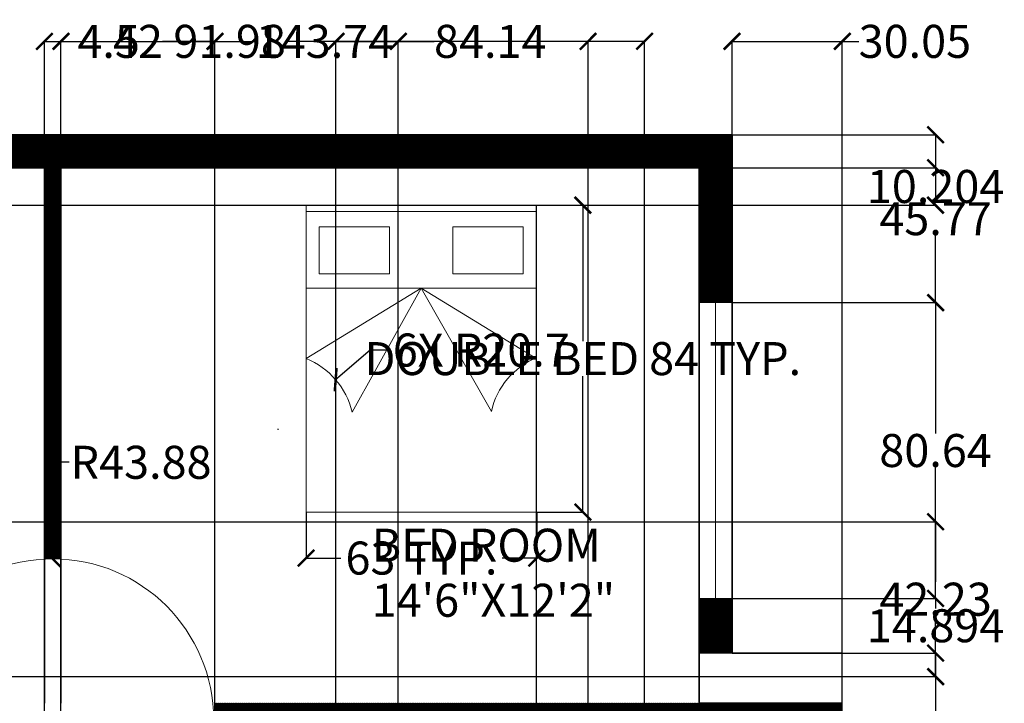
# Model space of a CAD drawing. Units: inches. Extents: x -43 to 552, y 22 to 537.
# Tile 4 of 4: x 283 to 552, y 351 to 537. Entities that reach past the tile are written whole.
import ezdxf

# ---------------------------------------------------------------- set-up
doc = ezdxf.new("R2010")
doc.units = ezdxf.units.IN
doc.header["$MEASUREMENT"] = 0
for name, color, linetype, lineweight in [('A-ANNO-DIMS', 2, 'Continuous', 18), ('A-AREA-IDEN', 7, 'Continuous', 18), ('A-DOOR', 4, 'Continuous', 18), ('A-FLOR', 7, 'Continuous', 25), ('A-FURN', 8, 'Continuous', 18), ('A-GLAZ', 4, 'Continuous', 18), ('A-WALL', 7, 'Continuous', 35), ('A-WALL-PATT', 252, 'Continuous', 13)]:
    doc.layers.add(name, color=color, linetype=linetype, lineweight=lineweight)
doc.styles.get("Standard").update_dxf_attribs({"font": 'arial.ttf'})
doc.dimstyles.get("Standard").update_dxf_attribs({"dimtxt": 9, "dimasz": 4.5, "dimexe": 0.18, "dimexo": 0.0625, "dimgap": 0.09, "dimtad": 0, "dimtih": 1, "dimtoh": 1, "dimdec": 1, "dimzin": 0, "dimdsep": 46, "dimlunit": 4, "dimtxsty": 'Standard', "dimblk": 'ARCHTICK', "dimcen": 0.09, "dimadec": 0, "dimazin": 0, "dimtfac": 1, "dimtdec": 1, "dimtofl": 0, "dimtmove": 0, "dimatfit": 3, "dimfxl": 1, "dimtolj": 1, "dimtzin": 0, "dimarcsym": 0})
pattern_1 = [(45, (-523.11303, 0), (-0.088388348, 0.088388348), [])]

# ---------------------------------------------------------------- blocks, each defined once
blk = doc.blocks.new('BED-DOUBLE')
for p, q in [((0, 83.65), (62.74, 83.65)), ((0, 0), (0, 83.65)), ((62.74, 83.65), (62.74, 0)), ((0, 81.91), (62.74, 81.91)), ((0, 61), (62.74, 61)), ((31.37, 61), (0, 41.83)), ((12.53, 27.23), (31.37, 61)), ((62.74, 41.83), (31.37, 61)), ((31.37, 61), (50.51, 27.4)), ((62.74, 0), (0, 0))]:
    blk.add_line(p, q)
for points in [[(3.55, 77.79), (22.76, 77.79), (22.76, 64.95), (3.55, 64.95)], [(59.19, 77.79), (39.98, 77.79), (39.98, 64.95), (59.19, 64.95)]]:
    blk.add_lwpolyline(points, close=True)
for centre, start, end in [((-7.65, 22.59), 12.9482, 68.3142), ((70.73, 22.94), 112.1918, 167.5578)]:
    blk.add_arc(centre, 20.7, start, end)
blk = doc.blocks.new('_ArchTick')
at = {"color": 0, "linetype": 'ByBlock', "const_width": 0.15}
blk.add_lwpolyline([(-0.5, -0.5), (0.5, 0.5)], dxfattribs=at)
blk = doc.blocks.new('*D4')
at = {"layer": 'A-ANNO-DIMS', "color": 0, "lineweight": -2, "transparency": 16777216}
for p, q in [((424.33, 486.74), (437, 486.74)), ((436.82, 486.74), (436.82, 449.66)), ((436.82, 403.09), (436.82, 440.17)), ((424.33, 403.09), (437, 403.09))]:
    blk.add_line(p, q, dxfattribs=at)
at = {"layer": 'Defpoints', "color": 0, "transparency": 16777216}
for p in [(424.27, 486.74), (436.82, 486.74), (424.27, 403.09)]:
    blk.add_point(p, dxfattribs=at)
at = {"layer": 'A-ANNO-DIMS', "color": 0, "lineweight": -2, "transparency": 16777216, "xscale": 4.5, "yscale": 4.5, "zscale": 4.5}
for p, rotation in [((436.82, 486.74), 90), ((436.82, 403.09), 270)]:
    blk.add_blockref('_ArchTick', p, dxfattribs=dict(at, rotation=rotation))
at = {"layer": 'A-ANNO-DIMS', "color": 0, "transparency": 16777216, "insert": (436.82, 444.92), "char_height": 9, "attachment_point": 5}
blk.add_mtext('\\A1;DOUBLE BED 84 TYP.', dxfattribs=at)
blk = doc.blocks.new('*D5')
at = {"layer": 'A-ANNO-DIMS', "color": 0, "lineweight": -2, "transparency": 16777216}
for p, q in [((361.36, 403.03), (361.36, 390.36)), ((424.27, 403.03), (424.27, 390.36)), ((361.36, 390.54), (370.8, 390.54)), ((424.27, 390.54), (414.84, 390.54))]:
    blk.add_line(p, q, dxfattribs=at)
at = {"layer": 'Defpoints', "color": 0, "transparency": 16777216}
for p in [(361.36, 403.09), (424.27, 403.09), (424.27, 390.54)]:
    blk.add_point(p, dxfattribs=at)
at = {"layer": 'A-ANNO-DIMS', "color": 0, "lineweight": -2, "transparency": 16777216, "xscale": 4.5, "yscale": 4.5, "zscale": 4.5, "rotation": 180}
blk.add_blockref('_ArchTick', (361.36, 390.54), dxfattribs=at)
at = {"layer": 'A-ANNO-DIMS', "color": 0, "lineweight": -2, "transparency": 16777216, "xscale": 4.5, "yscale": 4.5, "zscale": 4.5}
blk.add_blockref('_ArchTick', (424.27, 390.54), dxfattribs=at)
at = {"layer": 'A-ANNO-DIMS', "color": 0, "transparency": 16777216, "insert": (392.82, 390.54), "char_height": 9, "attachment_point": 5}
blk.add_mtext('\\A1;63 TYP.', dxfattribs=at)
blk = doc.blocks.new('*D9')
at = {"layer": 'A-ANNO-DIMS', "color": 0, "lineweight": -2, "transparency": 16777216}
for p, q in [((82.45, 505.95), (-24.17, 505.95)), ((-23.99, 505.95), (-23.99, 287.55)), ((-23.99, 59.77), (-23.99, 278.18)), ((289.95, 59.77), (-24.17, 59.77))]:
    blk.add_line(p, q, dxfattribs=at)
at = {"layer": 'Defpoints', "color": 0, "transparency": 16777216}
for p in [(-23.99, 505.95), (82.51, 505.95), (290.01, 59.77)]:
    blk.add_point(p, dxfattribs=at)
at = {"layer": 'A-ANNO-DIMS', "color": 0, "lineweight": -2, "transparency": 16777216, "xscale": 4.5, "yscale": 4.5, "zscale": 4.5}
for p, rotation in [((-23.99, 505.95), 90), ((-23.99, 59.77), 270)]:
    blk.add_blockref('_ArchTick', p, dxfattribs=dict(at, rotation=rotation))
at = {"layer": 'A-ANNO-DIMS', "color": 0, "transparency": 16777216, "insert": (-23.99, 282.86), "char_height": 9, "attachment_point": 5}
blk.add_mtext('\\A1;446.2', dxfattribs=at)
blk = doc.blocks.new('*D15')
at = {"layer": 'A-ANNO-DIMS', "color": 0, "lineweight": -2, "transparency": 16777216}
for p, q in [((477.51, 506.01), (477.51, 531.58)), ((477.51, 531.4), (507.56, 531.4)), ((507.56, 364.71), (507.56, 531.58)), ((507.56, 531.4), (512.06, 531.4))]:
    blk.add_line(p, q, dxfattribs=at)
at = {"layer": 'Defpoints', "color": 0, "transparency": 16777216}
for p in [(507.56, 531.4), (477.51, 505.95), (507.56, 364.65)]:
    blk.add_point(p, dxfattribs=at)
at = {"layer": 'A-ANNO-DIMS', "color": 0, "lineweight": -2, "transparency": 16777216, "xscale": 4.5, "yscale": 4.5, "zscale": 4.5, "rotation": 180}
blk.add_blockref('_ArchTick', (477.51, 531.4), dxfattribs=at)
at = {"layer": 'A-ANNO-DIMS', "color": 0, "lineweight": -2, "transparency": 16777216, "xscale": 4.5, "yscale": 4.5, "zscale": 4.5}
blk.add_blockref('_ArchTick', (507.56, 531.4), dxfattribs=at)
at = {"layer": 'A-ANNO-DIMS', "color": 0, "transparency": 16777216, "insert": (527.37, 531.4), "char_height": 9, "attachment_point": 5}
blk.add_mtext('\\A1;30.05', dxfattribs=at)
blk = doc.blocks.new('*D16')
at = {"layer": 'A-ANNO-DIMS', "color": 0, "lineweight": -2, "transparency": 16777216}
for p, q in [((477.57, 460.18), (533.19, 460.18)), ((533.01, 460.18), (533.01, 424.54)), ((533.01, 379.54), (533.01, 415.17)), ((477.57, 379.54), (533.19, 379.54))]:
    blk.add_line(p, q, dxfattribs=at)
at = {"layer": 'Defpoints', "color": 0, "transparency": 16777216}
for p in [(477.51, 460.18), (533.01, 460.18), (477.51, 379.54)]:
    blk.add_point(p, dxfattribs=at)
at = {"layer": 'A-ANNO-DIMS', "color": 0, "lineweight": -2, "transparency": 16777216, "xscale": 4.5, "yscale": 4.5, "zscale": 4.5}
for p, rotation in [((533.01, 460.18), 90), ((533.01, 379.54), 270)]:
    blk.add_blockref('_ArchTick', p, dxfattribs=dict(at, rotation=rotation))
at = {"layer": 'A-ANNO-DIMS', "color": 0, "transparency": 16777216, "insert": (533.01, 419.86), "char_height": 9, "attachment_point": 5}
blk.add_mtext('\\A1;80.64', dxfattribs=at)
blk = doc.blocks.new('*D17')
at = {"layer": 'A-ANNO-DIMS', "color": 0, "lineweight": -2, "transparency": 16777216}
for p, q in [((477.57, 505.95), (533.19, 505.95)), ((533.01, 505.95), (533.01, 487.73)), ((533.01, 460.18), (533.01, 478.39)), ((477.57, 460.18), (533.19, 460.18))]:
    blk.add_line(p, q, dxfattribs=at)
at = {"layer": 'Defpoints', "color": 0, "transparency": 16777216}
for p in [(477.51, 505.95), (533.01, 505.95), (477.51, 460.18)]:
    blk.add_point(p, dxfattribs=at)
at = {"layer": 'A-ANNO-DIMS', "color": 0, "lineweight": -2, "transparency": 16777216, "xscale": 4.5, "yscale": 4.5, "zscale": 4.5}
for p, rotation in [((533.01, 505.95), 90), ((533.01, 460.18), 270)]:
    blk.add_blockref('_ArchTick', p, dxfattribs=dict(at, rotation=rotation))
at = {"layer": 'A-ANNO-DIMS', "color": 0, "transparency": 16777216, "insert": (533.01, 483.06), "char_height": 9, "attachment_point": 5}
blk.add_mtext('\\A1;45.77', dxfattribs=at)
blk = doc.blocks.new('*D18')
at = {"layer": 'A-ANNO-DIMS', "color": 0, "lineweight": -2, "transparency": 16777216}
for p, q in [((477.57, 379.54), (533.19, 379.54)), ((533.01, 379.54), (533.01, 376.78)), ((533.01, 364.65), (533.01, 367.41)), ((477.57, 364.65), (533.19, 364.65))]:
    blk.add_line(p, q, dxfattribs=at)
at = {"layer": 'Defpoints', "color": 0, "transparency": 16777216}
for p in [(477.51, 379.54), (533.01, 379.54), (477.51, 364.65)]:
    blk.add_point(p, dxfattribs=at)
at = {"layer": 'A-ANNO-DIMS', "color": 0, "lineweight": -2, "transparency": 16777216, "xscale": 4.5, "yscale": 4.5, "zscale": 4.5}
for p, rotation in [((533.01, 379.54), 90), ((533.01, 364.65), 270)]:
    blk.add_blockref('_ArchTick', p, dxfattribs=dict(at, rotation=rotation))
at = {"layer": 'A-ANNO-DIMS', "color": 0, "transparency": 16777216, "insert": (533.01, 372.09), "char_height": 9, "attachment_point": 5}
blk.add_mtext('\\A1;14.894', dxfattribs=at)
blk = doc.blocks.new('*D19')
at = {"layer": 'A-ANNO-DIMS', "color": 0, "lineweight": -2, "transparency": 16777216}
for p, q in [((507.62, 364.65), (533.19, 364.65)), ((533.01, 364.65), (533.01, 297.15)), ((533.01, 220.29), (533.01, 287.78)), ((507.62, 220.29), (533.19, 220.29))]:
    blk.add_line(p, q, dxfattribs=at)
at = {"layer": 'Defpoints', "color": 0, "transparency": 16777216}
for p in [(507.56, 364.65), (533.01, 364.65), (507.56, 220.29)]:
    blk.add_point(p, dxfattribs=at)
at = {"layer": 'A-ANNO-DIMS', "color": 0, "lineweight": -2, "transparency": 16777216, "xscale": 4.5, "yscale": 4.5, "zscale": 4.5}
for p, rotation in [((533.01, 364.65), 90), ((533.01, 220.29), 270)]:
    blk.add_blockref('_ArchTick', p, dxfattribs=dict(at, rotation=rotation))
at = {"layer": 'A-ANNO-DIMS', "color": 0, "transparency": 16777216, "insert": (533.01, 292.47), "char_height": 9, "attachment_point": 5}
blk.add_mtext('\\A1;144.36', dxfattribs=at)
blk = doc.blocks.new('*D28')
at = {"layer": 'A-ANNO-DIMS', "color": 0, "lineweight": -2, "transparency": 16777216}
for p, q in [((369.51, 297.17), (369.51, 531.58)), ((369.51, 531.4), (396.32, 531.4)), ((453.65, 531.4), (426.84, 531.4)), ((453.65, 297.17), (453.65, 531.58))]:
    blk.add_line(p, q, dxfattribs=at)
at = {"layer": 'Defpoints', "color": 0, "transparency": 16777216}
for p in [(453.65, 531.4), (369.51, 297.11), (453.65, 297.11)]:
    blk.add_point(p, dxfattribs=at)
at = {"layer": 'A-ANNO-DIMS', "color": 0, "lineweight": -2, "transparency": 16777216, "xscale": 4.5, "yscale": 4.5, "zscale": 4.5, "rotation": 180}
blk.add_blockref('_ArchTick', (369.51, 531.4), dxfattribs=at)
at = {"layer": 'A-ANNO-DIMS', "color": 0, "lineweight": -2, "transparency": 16777216, "xscale": 4.5, "yscale": 4.5, "zscale": 4.5}
blk.add_blockref('_ArchTick', (453.65, 531.4), dxfattribs=at)
at = {"layer": 'A-ANNO-DIMS', "color": 0, "transparency": 16777216, "insert": (411.58, 531.4), "char_height": 9, "attachment_point": 5}
blk.add_mtext('\\A1;84.14', dxfattribs=at)
blk = doc.blocks.new('*D32')
at = {"layer": 'A-ANNO-DIMS', "color": 0, "lineweight": -2, "transparency": 16777216}
for p, q in [((290.01, 255.18), (290.01, 531.58)), ((290.01, 531.4), (294.51, 531.4)), ((294.51, 255.18), (294.51, 531.58)), ((294.51, 531.4), (299.01, 531.4))]:
    blk.add_line(p, q, dxfattribs=at)
at = {"layer": 'Defpoints', "color": 0, "transparency": 16777216}
for p in [(294.51, 531.4), (290.01, 255.12), (294.51, 255.12)]:
    blk.add_point(p, dxfattribs=at)
at = {"layer": 'A-ANNO-DIMS', "color": 0, "lineweight": -2, "transparency": 16777216, "xscale": 4.5, "yscale": 4.5, "zscale": 4.5, "rotation": 180}
blk.add_blockref('_ArchTick', (290.01, 531.4), dxfattribs=at)
at = {"layer": 'A-ANNO-DIMS', "color": 0, "lineweight": -2, "transparency": 16777216, "xscale": 4.5, "yscale": 4.5, "zscale": 4.5}
blk.add_blockref('_ArchTick', (294.51, 531.4), dxfattribs=at)
at = {"layer": 'A-ANNO-DIMS', "color": 0, "transparency": 16777216, "insert": (307.51, 531.4), "char_height": 9, "attachment_point": 5}
blk.add_mtext('\\A1;4.5', dxfattribs=at)
blk = doc.blocks.new('*D33')
at = {"layer": 'A-ANNO-DIMS', "color": 0, "lineweight": -2, "transparency": 16777216}
for p, q in [((294.51, 59.84), (294.51, 531.58)), ((294.51, 531.4), (348.05, 531.4)), ((438.25, 531.4), (384.71, 531.4)), ((438.25, 59.84), (438.25, 531.58))]:
    blk.add_line(p, q, dxfattribs=at)
at = {"layer": 'Defpoints', "color": 0, "transparency": 16777216}
for p in [(438.25, 531.4), (294.51, 59.77), (438.25, 59.77)]:
    blk.add_point(p, dxfattribs=at)
at = {"layer": 'A-ANNO-DIMS', "color": 0, "lineweight": -2, "transparency": 16777216, "xscale": 4.5, "yscale": 4.5, "zscale": 4.5, "rotation": 180}
blk.add_blockref('_ArchTick', (294.51, 531.4), dxfattribs=at)
at = {"layer": 'A-ANNO-DIMS', "color": 0, "lineweight": -2, "transparency": 16777216, "xscale": 4.5, "yscale": 4.5, "zscale": 4.5}
blk.add_blockref('_ArchTick', (438.25, 531.4), dxfattribs=at)
at = {"layer": 'A-ANNO-DIMS', "color": 0, "transparency": 16777216, "insert": (366.38, 531.4), "char_height": 9, "attachment_point": 5}
blk.add_mtext('\\A1;143.74', dxfattribs=at)
blk = doc.blocks.new('*D36')
at = {"layer": 'A-ANNO-DIMS', "color": 0, "lineweight": -2, "transparency": 16777216}
for p, q in [((82.57, 400.45), (533.19, 400.45)), ((533.01, 400.45), (533.01, 384.02)), ((533.01, 358.22), (533.01, 374.64)), ((82.57, 358.22), (533.19, 358.22))]:
    blk.add_line(p, q, dxfattribs=at)
at = {"layer": 'Defpoints', "color": 0, "transparency": 16777216}
for p in [(82.51, 400.45), (533.01, 400.45), (82.51, 358.22)]:
    blk.add_point(p, dxfattribs=at)
at = {"layer": 'A-ANNO-DIMS', "color": 0, "lineweight": -2, "transparency": 16777216, "xscale": 4.5, "yscale": 4.5, "zscale": 4.5}
for p, rotation in [((533.01, 400.45), 90), ((533.01, 358.22), 270)]:
    blk.add_blockref('_ArchTick', p, dxfattribs=dict(at, rotation=rotation))
at = {"layer": 'A-ANNO-DIMS', "color": 0, "transparency": 16777216, "insert": (533.01, 379.33), "char_height": 9, "attachment_point": 5}
blk.add_mtext('\\A1;42.23', dxfattribs=at)
blk = doc.blocks.new('*D38')
at = {"layer": 'A-ANNO-DIMS', "color": 0, "lineweight": -2, "transparency": 16777216}
for p, q in [((294.51, 243.34), (294.51, 531.58)), ((294.51, 531.4), (308.84, 531.4)), ((336.51, 531.4), (322.18, 531.4)), ((336.51, 243.34), (336.51, 531.58))]:
    blk.add_line(p, q, dxfattribs=at)
at = {"layer": 'Defpoints', "color": 0, "transparency": 16777216}
for p in [(336.51, 531.4), (294.51, 243.27), (336.51, 243.27)]:
    blk.add_point(p, dxfattribs=at)
at = {"layer": 'A-ANNO-DIMS', "color": 0, "lineweight": -2, "transparency": 16777216, "xscale": 4.5, "yscale": 4.5, "zscale": 4.5, "rotation": 180}
blk.add_blockref('_ArchTick', (294.51, 531.4), dxfattribs=at)
at = {"layer": 'A-ANNO-DIMS', "color": 0, "lineweight": -2, "transparency": 16777216, "xscale": 4.5, "yscale": 4.5, "zscale": 4.5}
blk.add_blockref('_ArchTick', (336.51, 531.4), dxfattribs=at)
at = {"layer": 'A-ANNO-DIMS', "color": 0, "transparency": 16777216, "insert": (315.51, 531.4), "char_height": 9, "attachment_point": 5}
blk.add_mtext('\\A1;42', dxfattribs=at)
blk = doc.blocks.new('*D40')
at = {"layer": 'A-ANNO-DIMS', "color": 0, "lineweight": -2, "transparency": 16777216}
for p, q in [((197.07, 496.95), (533.19, 496.95)), ((533.01, 496.95), (533.01, 496.53)), ((192.25, 486.74), (533.19, 486.74)), ((533.01, 486.74), (533.01, 487.16))]:
    blk.add_line(p, q, dxfattribs=at)
at = {"layer": 'Defpoints', "color": 0, "transparency": 16777216}
for p in [(197.01, 496.95), (533.01, 496.95), (192.19, 486.74)]:
    blk.add_point(p, dxfattribs=at)
at = {"layer": 'A-ANNO-DIMS', "color": 0, "lineweight": -2, "transparency": 16777216, "xscale": 4.5, "yscale": 4.5, "zscale": 4.5}
for p, rotation in [((533.01, 496.95), 90), ((533.01, 486.74), 270)]:
    blk.add_blockref('_ArchTick', p, dxfattribs=dict(at, rotation=rotation))
at = {"layer": 'A-ANNO-DIMS', "color": 0, "transparency": 16777216, "insert": (533.01, 491.84), "char_height": 9, "attachment_point": 5}
blk.add_mtext('\\A1;10.204', dxfattribs=at)
blk = doc.blocks.new('*D41')
at = {"layer": 'A-ANNO-DIMS', "color": 0, "lineweight": -2, "transparency": 16777216}
for p, q in [((468.51, 496.88), (468.51, 34.14)), ((424.1, 486.68), (424.1, 34.14)), ((424.1, 34.32), (431.72, 34.32)), ((468.51, 34.32), (460.89, 34.32))]:
    blk.add_line(p, q, dxfattribs=at)
at = {"layer": 'Defpoints', "color": 0, "transparency": 16777216}
for p in [(468.51, 496.95), (424.1, 486.74), (468.51, 34.32)]:
    blk.add_point(p, dxfattribs=at)
at = {"layer": 'A-ANNO-DIMS', "color": 0, "lineweight": -2, "transparency": 16777216, "xscale": 4.5, "yscale": 4.5, "zscale": 4.5, "rotation": 180}
blk.add_blockref('_ArchTick', (424.1, 34.32), dxfattribs=at)
at = {"layer": 'A-ANNO-DIMS', "color": 0, "lineweight": -2, "transparency": 16777216, "xscale": 4.5, "yscale": 4.5, "zscale": 4.5}
blk.add_blockref('_ArchTick', (468.51, 34.32), dxfattribs=at)
at = {"layer": 'A-ANNO-DIMS', "color": 0, "transparency": 16777216, "insert": (446.31, 34.32), "char_height": 9, "attachment_point": 5}
blk.add_mtext('\\A1;44.41', dxfattribs=at)
blk = doc.blocks.new('*D42')
at = {"layer": 'A-ANNO-DIMS', "color": 0, "lineweight": -2, "transparency": 16777216}
for p, q in [((294.51, 116.84), (294.51, 531.58)), ((294.51, 531.4), (325.22, 531.4)), ((386.5, 531.4), (355.79, 531.4)), ((386.5, 150.32), (386.5, 531.58))]:
    blk.add_line(p, q, dxfattribs=at)
at = {"layer": 'Defpoints', "color": 0, "transparency": 16777216}
for p in [(386.5, 531.4), (386.5, 150.25), (294.51, 116.77)]:
    blk.add_point(p, dxfattribs=at)
at = {"layer": 'A-ANNO-DIMS', "color": 0, "lineweight": -2, "transparency": 16777216, "xscale": 4.5, "yscale": 4.5, "zscale": 4.5, "rotation": 180}
blk.add_blockref('_ArchTick', (294.51, 531.4), dxfattribs=at)
at = {"layer": 'A-ANNO-DIMS', "color": 0, "lineweight": -2, "transparency": 16777216, "xscale": 4.5, "yscale": 4.5, "zscale": 4.5}
blk.add_blockref('_ArchTick', (386.5, 531.4), dxfattribs=at)
at = {"layer": 'A-ANNO-DIMS', "color": 0, "transparency": 16777216, "insert": (340.5, 531.4), "char_height": 9, "attachment_point": 5}
blk.add_mtext('\\A1;91.98', dxfattribs=at)
blk = doc.blocks.new('*D55')
at = {"layer": 'A-ANNO-DIMS', "color": 0, "lineweight": -2, "transparency": 16777216}
for p, q in [((296.76, 416.65), (292.26, 416.65)), ((292.26, 416.65), (292.26, 390.33)), ((292.17, 346.45), (292.35, 346.45)), ((292.26, 346.36), (292.26, 346.54))]:
    blk.add_line(p, q, dxfattribs=at)
at = {"layer": 'Defpoints', "color": 0, "transparency": 16777216}
for p in [(292.26, 390.33), (292.26, 346.45)]:
    blk.add_point(p, dxfattribs=at)
at = {"layer": 'A-ANNO-DIMS', "color": 0, "lineweight": -2, "transparency": 16777216, "xscale": 4.5, "yscale": 4.5, "zscale": 4.5, "rotation": 269.9994946781158}
blk.add_blockref('_ArchTick', (292.26, 390.33), dxfattribs=at)
at = {"layer": 'A-ANNO-DIMS', "color": 0, "transparency": 16777216, "insert": (316.35, 416.65), "char_height": 9, "attachment_point": 5}
blk.add_mtext('\\A1;R43.88', dxfattribs=at)
blk = doc.blocks.new('*D58')
at = {"layer": 'A-ANNO-DIMS', "color": 0, "lineweight": -2, "transparency": 16777216}
for p, q in [((378.85, 447.25), (369.42, 439.16)), ((383.35, 447.25), (378.85, 447.25)), ((353.62, 425.68), (353.8, 425.68)), ((353.71, 425.59), (353.71, 425.77))]:
    blk.add_line(p, q, dxfattribs=at)
at = {"layer": 'Defpoints', "color": 0, "transparency": 16777216}
for p in [(369.42, 439.16), (353.71, 425.68)]:
    blk.add_point(p, dxfattribs=at)
at = {"layer": 'A-ANNO-DIMS', "color": 0, "lineweight": -2, "transparency": 16777216, "xscale": 4.5, "yscale": 4.5, "zscale": 4.5, "rotation": 220.6315320270985}
blk.add_blockref('_ArchTick', (369.42, 439.16), dxfattribs=at)
at = {"layer": 'A-ANNO-DIMS', "color": 0, "transparency": 16777216, "insert": (409.13, 447.25), "char_height": 9, "attachment_point": 5}
blk.add_mtext('\\A1;6X R20.7', dxfattribs=at)

msp = doc.modelspace()

# ---------------------------------------------------------------- hatches: boundary and pattern name
at = {"layer": 'A-WALL-PATT'}
h = msp.add_hatch(dxfattribs=at)
h.set_pattern_fill('ANSI31', color=256)
h.set_pattern_definition(pattern_1)
h.paths.add_polyline_path([(202.9985, 146.4471), (169.965, 146.4471), (169.965, 255.1157), (165.465, 255.1157), (165.465, 146.4471), (147.9805, 146.4471), (147.9805, 141.9471), (165.465, 141.9471), (165.465, 84.9471), (169.965, 84.9471), (169.965, 141.9471), (202.9985, 141.9471)])
h.paths.add_polyline_path([(294.5106, 146.4471), (294.5106, 238.775), (294.5106, 243.275), (294.5106, 255.1157), (290.0106, 255.1157), (290.0106, 146.4471), (247.8411, 146.4471), (247.8411, 141.9471), (290.0106, 141.9471), (290.0106, 93.9471), (290.0106, 59.775), (294.5106, 59.775), (294.5106, 77.3814), (294.5106, 93.9471), (294.5106, 107.775), (316.2676, 107.775), (316.2676, 116.775), (294.5106, 116.775)])
h.paths.add_polyline_path([(10.465, 346.4471), (82.5106, 346.4471), (91.5106, 346.4471), (91.5106, 358.2163), (82.5106, 358.2163), (82.5106, 350.9471), (1.465, 350.9471), (1.465, 84.9471), (10.465, 84.9471), (10.465, 141.9471), (56.4237, 141.9471), (56.4237, 146.4471), (10.465, 146.4471)])
h.paths.add_polyline_path([(91.5106, 496.9471), (107.5106, 496.9471), (107.5106, 505.9471), (82.5106, 505.9471), (82.5106, 400.4471), (147.5106, 400.4471), (147.5106, 346.4471), (248.0106, 346.4471), (248.0106, 350.9471), (152.0106, 350.9471), (152.0106, 496.9471), (197.0106, 496.9471), (197.0106, 505.9471), (131.5106, 505.9471), (131.5106, 496.9471), (147.5106, 496.9471), (147.5106, 404.9471), (91.5106, 404.9471)])
h.paths.add_polyline_path([(477.5106, 505.9471), (245.0106, 505.9471), (245.0106, 496.9471), (290.0106, 496.9471), (290.0106, 390.2693, -0.02565505), (294.5106, 390.2693), (294.5106, 496.9471), (468.5106, 496.9471), (468.5106, 460.1763), (477.5106, 460.1763)])
h = msp.add_hatch(dxfattribs=at)
h.set_pattern_fill('ANSI31', color=256)
h.set_pattern_definition(pattern_1)
h.paths.add_polyline_path([(462.6472, 350.9471), (453.6472, 350.9471), (453.6472, 243.275), (462.6472, 243.275)])
h.paths.add_polyline_path([(507.5611, 350.9471), (468.5106, 350.9471), (462.6472, 350.9471), (462.6472, 346.4471), (468.5106, 346.4471), (507.5611, 346.4471)])
h.paths.add_polyline_path([(453.6472, 350.9471), (336.5106, 350.9471), (336.5106, 346.4471), (453.6472, 346.4471)])
h.paths.add_polyline_path([(477.5106, 137.2859), (468.5106, 137.2859), (468.5106, 116.775), (377.5838, 116.775), (377.5838, 107.775), (438.2457, 107.775), (438.2457, 59.775), (447.2457, 59.775), (447.2457, 107.775), (477.5106, 107.775)])
h.paths.add_polyline_path([(477.5106, 379.5395), (468.5106, 379.5395), (468.5106, 364.6452), (477.5106, 364.6452)])
h.paths.add_polyline_path([(477.5106, 238.775), (468.5106, 238.775), (468.5106, 220.2859), (477.5106, 220.2859)])
h.paths.add_polyline_path([(507.5611, 243.275), (468.5106, 243.275), (462.6472, 243.275), (462.6472, 238.775), (468.5106, 238.775), (477.5106, 238.775), (507.5611, 238.775)])
h.paths.add_polyline_path([(462.6472, 243.275), (453.6472, 243.275), (453.6472, 238.775), (462.6472, 238.775)])
h.paths.add_polyline_path([(453.6472, 243.275), (369.5106, 243.275), (369.5106, 292.6111), (453.6472, 292.6111), (453.6472, 297.1111), (369.5106, 297.1111), (369.5106, 346.4471), (365.0106, 346.4471), (365.0106, 243.275), (336.5106, 243.275), (336.5106, 238.775), (453.6472, 238.775)])

# ---------------------------------------------------------------- linework, layer by layer
at = {"layer": 'A-DOOR'}
msp.add_arc((292.2606, 346.4471), 43.8799, 0, 180, dxfattribs=at)
at = {"layer": 'A-FLOR'}
for p, q in [((507.5611, 364.6452), (468.5106, 364.6452)), ((507.5611, 220.2859), (507.5611, 364.6452))]:
    msp.add_line(p, q, dxfattribs=at)
at = {"layer": 'A-GLAZ'}
for p, q in [((468.5106, 460.1763), (477.5106, 460.1763)), ((473.0106, 460.1763), (473.0106, 379.5395)), ((468.5106, 379.5395), (477.5106, 379.5395))]:
    msp.add_line(p, q, dxfattribs=at)
at = {"layer": 'A-WALL'}
for p, q in [((82.5106, 505.9471), (477.5106, 505.9471)), ((477.5106, 505.9471), (477.5106, 364.6452)), ((152.0106, 496.9471), (290.0106, 496.9471)), ((290.0106, 496.9471), (290.0106, 350.9471)), ((294.5106, 496.9471), (294.5106, 350.9471)), ((294.5106, 496.9471), (468.5106, 496.9471)), ((468.5106, 496.9471), (468.5106, 350.9471)), ((468.5106, 350.9471), (507.5611, 350.9471))]:
    msp.add_line(p, q, dxfattribs=at)

# ---------------------------------------------------------------- block references
at = {"layer": 'A-FURN'}
msp.add_blockref('BED-DOUBLE', (361.3632, 403.0902), dxfattribs=at)

# ---------------------------------------------------------------- texts
at = {"layer": 'A-AREA-IDEN', "insert": (379.2354, 398.5401), "char_height": 9, "attachment_point": 1}
msp.add_mtext_dynamic_manual_height_columns('BED ROOM\\P14\'6"X12\'2"', width=549.697564, gutter_width=1, heights=[0], dxfattribs=at)

# ---------------------------------------------------------------- dimensions: what is measured, and where the dimension line sits
at = {"layer": 'A-ANNO-DIMS'}
for base, p1, p2, override, picture, middle in [((294.5106, 531.3971), (290.0106, 255.1157), (294.5106, 255.1157), {"dimdec": 1, "dimlfac": 1, "dimrnd": 0, "dimzin": 0, "dimdsep": 46, "dimlunit": 2}, '*D32', (307.5082, 531.3971)), ((438.2457, 531.3971), (294.5106, 59.775), (438.2457, 59.775), {"dimdec": 2, "dimlfac": 1, "dimrnd": 0, "dimzin": 0, "dimdsep": 46, "dimlunit": 2}, '*D33', (366.3781, 531.3971)), ((336.5106, 531.3971), (294.5106, 243.275), (336.5106, 243.275), {"dimdec": 0, "dimlfac": 1, "dimrnd": 0, "dimzin": 0, "dimdsep": 46, "dimlunit": 2}, '*D38', (315.5106, 531.3971)), ((386.4952, 531.3971), (294.5106, 116.775), (386.4952, 150.2529), {"dimdec": 2, "dimlfac": 1, "dimrnd": 0, "dimzin": 0, "dimdsep": 46, "dimlunit": 2}, '*D42', (340.5029, 531.3971)), ((453.6472, 531.3971), (369.5106, 297.1111), (453.6472, 297.1111), {"dimdec": 2, "dimlfac": 1, "dimrnd": 0, "dimzin": 0, "dimdsep": 46, "dimlunit": 2}, '*D28', (411.5789, 531.3971)), ((507.5611, 531.3971), (477.5106, 505.9471), (507.5611, 364.6452), {"dimdec": 2, "dimlfac": 1, "dimrnd": 0, "dimzin": 0, "dimdsep": 46, "dimlunit": 2}, '*D15', (527.367, 531.3971)), ((468.5106, 34.325), (424.1025, 486.7427), (468.5106, 496.9471), {"dimdec": 2, "dimlfac": 1, "dimrnd": 0, "dimzin": 0, "dimdsep": 46, "dimlunit": 2}, '*D41', (446.3066, 34.325))]:
    dim = msp.add_linear_dim(base=base, p1=p1, p2=p2, dimstyle='Standard', override=override, dxfattribs=at)
    dim.commit()
    dim.dimension.update_dxf_attribs({"geometry": picture, "text_midpoint": middle})
for base, p1, p2, override, picture, middle in [((-23.985, 505.9471), (290.0106, 59.775), (82.5106, 505.9471), {"dimdec": 1, "dimlfac": 1, "dimrnd": 0, "dimzin": 0, "dimdsep": 46, "dimlunit": 2}, '*D9', (-23.985, 282.8611)), ((533.0111, 505.9471), (477.5106, 460.1763), (477.5106, 505.9471), {"dimdec": 2, "dimlfac": 1, "dimrnd": 0, "dimzin": 0, "dimdsep": 46, "dimlunit": 2}, '*D17', (533.0111, 483.0617)), ((533.0111, 496.9471), (192.1876, 486.7427), (197.0106, 496.9471), {"dimdec": 3, "dimlfac": 1, "dimrnd": 0, "dimzin": 0, "dimdsep": 46, "dimlunit": 2}, '*D40', (533.0111, 491.8449)), ((533.0111, 460.1763), (477.5106, 379.5395), (477.5106, 460.1763), {"dimdec": 2, "dimlfac": 1, "dimrnd": 0, "dimzin": 0, "dimdsep": 46, "dimlunit": 2}, '*D16', (533.0111, 419.8579)), ((533.0111, 400.4471), (82.5106, 358.2163), (82.5106, 400.4471), {"dimdec": 2, "dimlfac": 1, "dimrnd": 0, "dimzin": 0, "dimdsep": 46, "dimlunit": 2}, '*D36', (533.0111, 379.3317)), ((533.0111, 379.5395), (477.5106, 364.6452), (477.5106, 379.5395), {"dimdec": 3, "dimlfac": 1, "dimrnd": 0, "dimzin": 0, "dimdsep": 46, "dimlunit": 2}, '*D18', (533.0111, 372.0924)), ((533.0111, 364.6452), (507.5611, 220.2859), (507.5611, 364.6452), {"dimdec": 2, "dimlfac": 1, "dimrnd": 0, "dimzin": 0, "dimdsep": 46, "dimlunit": 2}, '*D19', (533.0111, 292.4656))]:
    dim = msp.add_linear_dim(base=base, p1=p1, p2=p2, angle=90, dimstyle='Standard', override=override, dxfattribs=at)
    dim.commit()
    dim.dimension.update_dxf_attribs({"geometry": picture, "text_midpoint": middle})
dim = msp.add_linear_dim(base=(436.8185, 486.7427), p1=(424.2706, 403.0902), p2=(424.2706, 486.7427), angle=90, text='DOUBLE BED <> TYP.', dimstyle='Standard', override={"dimdec": 0, "dimlfac": 1, "dimrnd": 0, "dimzin": 0, "dimdsep": 46, "dimlunit": 2}, dxfattribs=at)
dim.commit()
dim.dimension.update_dxf_attribs({"geometry": '*D4', "text_midpoint": (436.8185, 444.9164)})
dim = msp.add_radius_dim(center=(353.714, 425.6809), mpoint=(369.424, 439.161), text='6X <>', dimstyle='Standard', override={"dimdec": 1, "dimlfac": 1, "dimrnd": 0, "dimzin": 0, "dimdsep": 46, "dimlunit": 2}, dxfattribs=at)
dim.commit()
dim.dimension.update_dxf_attribs({"geometry": '*D58', "text_midpoint": (409.1293, 447.249), "dimtype": 164})
dim = msp.add_radius_dim(center=(292.2606, 346.4471), mpoint=(292.261, 390.327), dimstyle='Standard', override={"dimdec": 2, "dimlfac": 1, "dimrnd": 0, "dimzin": 0, "dimdsep": 46, "dimlunit": 2}, dxfattribs=at)
dim.commit()
dim.dimension.update_dxf_attribs({"geometry": '*D55', "text_midpoint": (316.3523, 416.655), "dimtype": 164})
dim = msp.add_linear_dim(base=(424.2706, 390.5423), p1=(361.3632, 403.0902), p2=(424.2706, 403.0902), text='<> TYP.', dimstyle='Standard', override={"dimdec": 0, "dimlfac": 1, "dimrnd": 0, "dimzin": 0, "dimdsep": 46, "dimlunit": 2}, dxfattribs=at)
dim.commit()
dim.dimension.update_dxf_attribs({"geometry": '*D5', "text_midpoint": (392.8169, 390.5423)})

doc.saveas('drawing.dxf')
